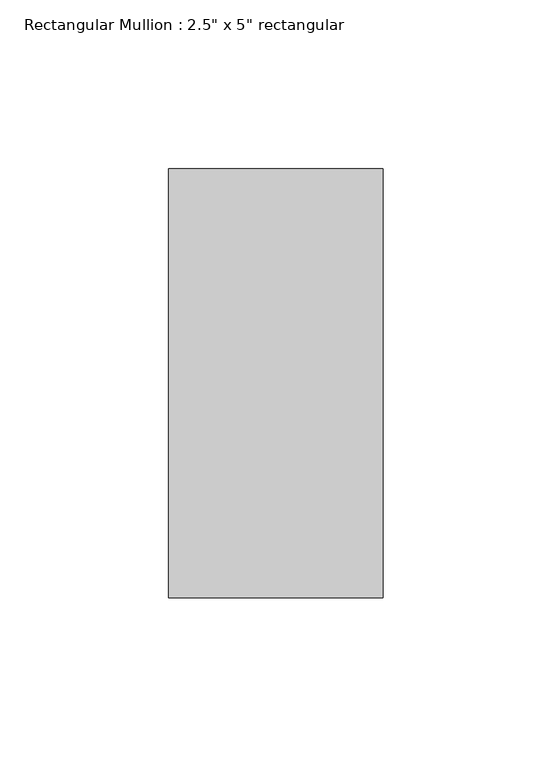
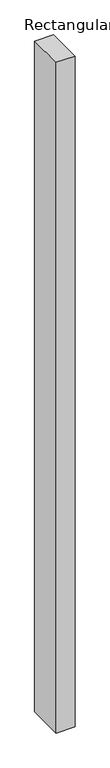
"""IFC4 building model written with IfcOpenShell, lengths in millimetres: member geometry."""

from ifc_helpers import new_model, si_unit, frame, origin, place, context, project, spatial, polyline, outline, extrude, source, transform, mapped, element, save


def member_6d59fc0e(model_context):
    return source(origin(), model_context, "Body", "SweptSolid", [
        extrude(outline(polyline([(0.0, 63.5), (0.0, -63.5), (-63.5, -63.5), (-63.5, 63.5), (0.0, 63.5)])), frame((0.0, 0.0, -2413.0), z_axis=(0.0, 0.0, 1.0), x_axis=(1.0, 0.0, 0.0)), (0.0, 0.0, 1.0), 2413.0),
    ])


if __name__ == "__main__":
    model = new_model("IFC4")
    model_context = context("Model", 3, world=origin())
    ifc_project = project(units=[si_unit("LENGTHUNIT", "METRE", prefix="MILLI")], contexts=[model_context])
    site = spatial("IfcSite", under=ifc_project)
    building = spatial("IfcBuilding", under=site)
    placement = place(None, origin())
    member_shape = member_6d59fc0e(model_context)
    element("IfcMember", 1, ObjectType="Rectangular Mullion : 2.5\" x 5\" rectangular", at=placement, inside=building, context=model_context, shape_type="MappedRepresentation", body=[
        mapped(member_shape, transform((0.0, 0.0, 0.0), x_axis=(1.0, 0.0, 0.0), y_axis=(0.0, 1.0, 0.0), z_axis=(0.0, 0.0, 1.0))),
    ])
    save(model, "model.ifc")

# Revit data of these elements
# Type "Rectangular Mullion : 2.5\" x 5\" rectangular"
#   built-in parameter 1007304 = 0.416667 (stored number, unit not read)
#   built-in parameter 1007301 = 0.104167 (stored number, unit not read)
#   built-in parameter 1007300 = 0.104167 (stored number, unit not read)
# Element 1 (IfcMember, "Rectangular Mullion : 2.5\" x 5\" rectangular")
#   Materials on its faces: "Aluminum"
# Materials
#   "Aluminum": class "Metal", colour RGB 247 247 247, transparency 0, Description = "Aluminum 6061", Cost = 0
